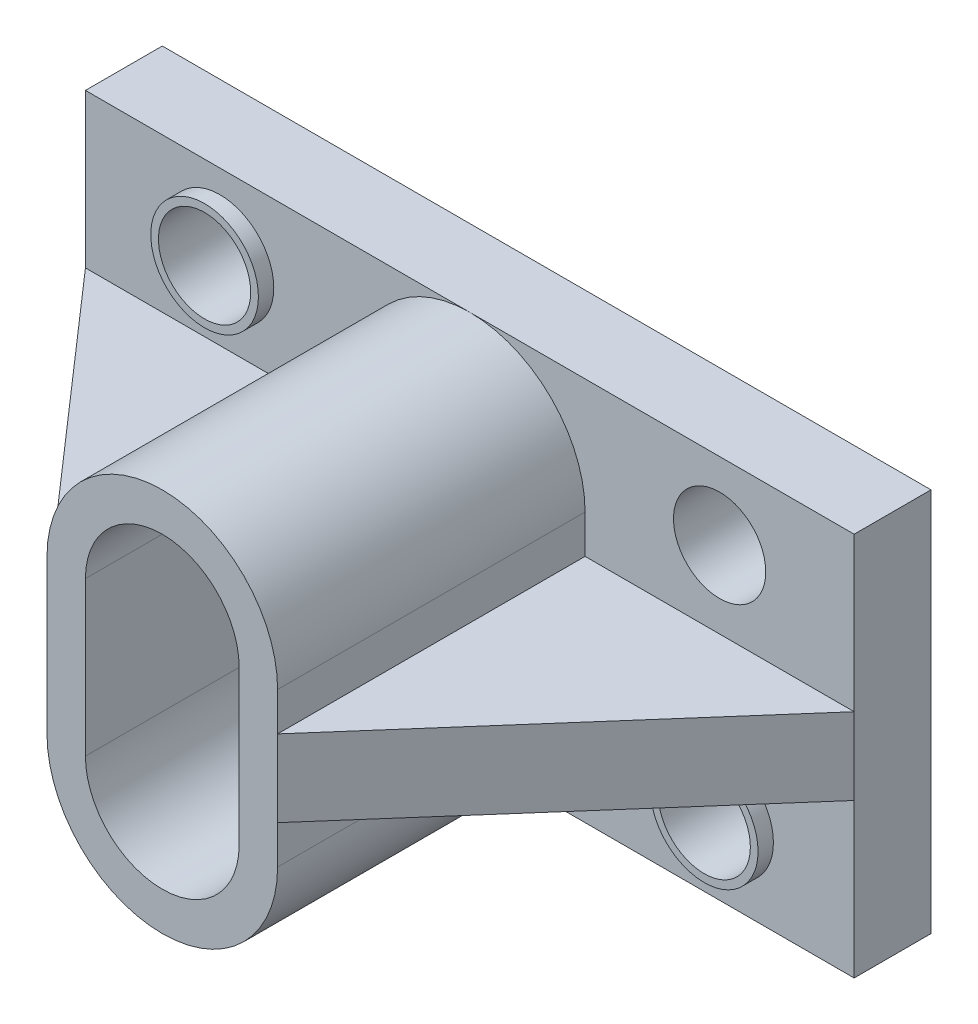
ISO-10303-21;
HEADER;
FILE_DESCRIPTION(('STEP AP214'),'2;1');
FILE_NAME('part.step','',(''),(''),'','','');
FILE_SCHEMA(('AUTOMOTIVE_DESIGN { 1 0 10303 214 1 1 1 1 }'));
ENDSEC;
DATA;
#1=APPLICATION_CONTEXT('core data for automotive mechanical design processes');
#2=APPLICATION_PROTOCOL_DEFINITION('international standard','automotive_design',2000,#1);
#3=PRODUCT_CONTEXT('',#1,'mechanical');
#4=PRODUCT('Part','Part','',(#3));
#5=PRODUCT_RELATED_PRODUCT_CATEGORY('part','',(#4));
#6=PRODUCT_DEFINITION_FORMATION('','',#4);
#7=PRODUCT_DEFINITION_CONTEXT('part definition',#1,'design');
#8=PRODUCT_DEFINITION('design','',#6,#7);
#9=PRODUCT_DEFINITION_SHAPE('','',#8);
#10=(LENGTH_UNIT() NAMED_UNIT(*) SI_UNIT(.MILLI.,.METRE.));
#11=(NAMED_UNIT(*) PLANE_ANGLE_UNIT() SI_UNIT($,.RADIAN.));
#12=(NAMED_UNIT(*) SI_UNIT($,.STERADIAN.) SOLID_ANGLE_UNIT());
#13=UNCERTAINTY_MEASURE_WITH_UNIT(LENGTH_MEASURE(1.E-05),#10,'distance_accuracy_value','');
#14=(GEOMETRIC_REPRESENTATION_CONTEXT(3) GLOBAL_UNCERTAINTY_ASSIGNED_CONTEXT((#13)) GLOBAL_UNIT_ASSIGNED_CONTEXT((#10,
#11,#12)) REPRESENTATION_CONTEXT('',''));
#15=CARTESIAN_POINT('',(0.,0.,0.));
#16=DIRECTION('',(0.,0.,1.));
#17=DIRECTION('',(1.,0.,0.));
#18=AXIS2_PLACEMENT_3D('',#15,#16,#17);
#19=CARTESIAN_POINT('',(0.,0.,10.));
#20=DIRECTION('',(0.,0.,1.));
#21=DIRECTION('',(1.,0.,0.));
#22=AXIS2_PLACEMENT_3D('',#19,#20,#21);
#23=PLANE('',#22);
#24=CARTESIAN_POINT('',(17.5,10.,10.));
#25=DIRECTION('',(0.,0.,1.));
#26=DIRECTION('',(1.,0.,0.));
#27=AXIS2_PLACEMENT_3D('',#24,#25,#26);
#28=CIRCLE('',#27,7.);
#29=CARTESIAN_POINT('',(24.5,10.,10.));
#30=VERTEX_POINT('',#29);
#31=EDGE_CURVE('E278',#30,#30,#28,.T.);
#32=ORIENTED_EDGE('',*,*,#31,.F.);
#33=EDGE_LOOP('',(#32));
#34=FACE_BOUND('',#33,.T.);
#35=DIRECTION('',(0.,-1.,0.));
#36=VECTOR('',#35,1.);
#37=CARTESIAN_POINT('',(35.,15.,10.));
#38=LINE('',#37,#36);
#39=CARTESIAN_POINT('',(35.,20.,10.));
#40=VERTEX_POINT('',#39);
#41=CARTESIAN_POINT('',(35.,15.,10.));
#42=VERTEX_POINT('',#41);
#43=EDGE_CURVE('E380',#40,#42,#38,.T.);
#44=ORIENTED_EDGE('',*,*,#43,.F.);
#45=DIRECTION('',(-1.,0.,0.));
#46=VECTOR('',#45,1.);
#47=CARTESIAN_POINT('',(0.,20.,10.));
#48=LINE('',#47,#46);
#49=CARTESIAN_POINT('',(0.,20.,10.));
#50=VERTEX_POINT('',#49);
#51=EDGE_CURVE('E72',#40,#50,#48,.T.);
#52=ORIENTED_EDGE('',*,*,#51,.T.);
#53=DIRECTION('',(0.,-1.,0.));
#54=VECTOR('',#53,1.);
#55=CARTESIAN_POINT('',(0.,50.,10.));
#56=LINE('',#55,#54);
#57=CARTESIAN_POINT('',(0.,0.,10.));
#58=VERTEX_POINT('',#57);
#59=EDGE_CURVE('E397',#50,#58,#56,.T.);
#60=ORIENTED_EDGE('',*,*,#59,.T.);
#61=DIRECTION('',(1.,0.,0.));
#62=VECTOR('',#61,1.);
#63=CARTESIAN_POINT('',(0.,0.,10.));
#64=LINE('',#63,#62);
#65=CARTESIAN_POINT('',(50.,0.,10.));
#66=VERTEX_POINT('',#65);
#67=EDGE_CURVE('E399',#58,#66,#64,.T.);
#68=ORIENTED_EDGE('',*,*,#67,.T.);
#69=CARTESIAN_POINT('',(50.,15.,10.));
#70=DIRECTION('',(0.,0.,1.));
#71=DIRECTION('',(1.,0.,0.));
#72=AXIS2_PLACEMENT_3D('',#69,#70,#71);
#73=CIRCLE('',#72,15.);
#74=EDGE_CURVE('E355',#42,#66,#73,.T.);
#75=ORIENTED_EDGE('',*,*,#74,.F.);
#76=EDGE_LOOP('',(#44,#52,#60,#68,#75));
#77=FACE_BOUND('',#76,.T.);
#78=ADVANCED_FACE('F44',(#34,#77),#23,.T.);
#79=CARTESIAN_POINT('',(35.,15.,50.));
#80=DIRECTION('',(1.,0.,0.));
#81=DIRECTION('',(0.,0.,-1.));
#82=AXIS2_PLACEMENT_3D('',#79,#80,#81);
#83=PLANE('',#82);
#84=DIRECTION('',(0.,0.,1.));
#85=VECTOR('',#84,1.);
#86=CARTESIAN_POINT('',(35.,20.,50.));
#87=LINE('',#86,#85);
#88=CARTESIAN_POINT('',(35.,20.,50.));
#89=VERTEX_POINT('',#88);
#90=EDGE_CURVE('E288',#40,#89,#87,.T.);
#91=ORIENTED_EDGE('',*,*,#90,.F.);
#92=ORIENTED_EDGE('',*,*,#43,.T.);
#93=DIRECTION('',(0.,0.,-1.));
#94=VECTOR('',#93,1.);
#95=CARTESIAN_POINT('',(35.,15.,50.));
#96=LINE('',#95,#94);
#97=CARTESIAN_POINT('',(35.,15.,50.));
#98=VERTEX_POINT('',#97);
#99=EDGE_CURVE('E367',#98,#42,#96,.T.);
#100=ORIENTED_EDGE('',*,*,#99,.F.);
#101=DIRECTION('',(0.,-1.,0.));
#102=VECTOR('',#101,1.);
#103=CARTESIAN_POINT('',(35.,15.,50.));
#104=LINE('',#103,#102);
#105=EDGE_CURVE('E362',#89,#98,#104,.T.);
#106=ORIENTED_EDGE('',*,*,#105,.F.);
#107=EDGE_LOOP('',(#91,#92,#100,#106));
#108=FACE_BOUND('',#107,.T.);
#109=ADVANCED_FACE('F450',(#108),#83,.F.);
#110=CARTESIAN_POINT('',(82.5,10.,10.));
#111=DIRECTION('',(0.,0.,1.));
#112=DIRECTION('',(1.,0.,0.));
#113=AXIS2_PLACEMENT_3D('',#110,#111,#112);
#114=CIRCLE('',#113,7.);
#115=CARTESIAN_POINT('',(89.5,10.,10.));
#116=VERTEX_POINT('',#115);
#117=EDGE_CURVE('E272',#116,#116,#114,.T.);
#118=ORIENTED_EDGE('',*,*,#117,.F.);
#119=EDGE_LOOP('',(#118));
#120=FACE_BOUND('',#119,.T.);
#121=DIRECTION('',(0.,1.,0.));
#122=VECTOR('',#121,1.);
#123=CARTESIAN_POINT('',(100.,0.,10.));
#124=LINE('',#123,#122);
#125=CARTESIAN_POINT('',(100.,0.,10.));
#126=VERTEX_POINT('',#125);
#127=CARTESIAN_POINT('',(100.,20.,10.));
#128=VERTEX_POINT('',#127);
#129=EDGE_CURVE('E402',#126,#128,#124,.T.);
#130=ORIENTED_EDGE('',*,*,#129,.T.);
#131=DIRECTION('',(-1.,0.,0.));
#132=VECTOR('',#131,1.);
#133=CARTESIAN_POINT('',(0.,20.,10.));
#134=LINE('',#133,#132);
#135=CARTESIAN_POINT('',(65.,20.,10.));
#136=VERTEX_POINT('',#135);
#137=EDGE_CURVE('E312',#128,#136,#134,.T.);
#138=ORIENTED_EDGE('',*,*,#137,.T.);
#139=DIRECTION('',(0.,1.,0.));
#140=VECTOR('',#139,1.);
#141=CARTESIAN_POINT('',(65.,15.,10.));
#142=LINE('',#141,#140);
#143=CARTESIAN_POINT('',(65.,15.,10.));
#144=VERTEX_POINT('',#143);
#145=EDGE_CURVE('E372',#144,#136,#142,.T.);
#146=ORIENTED_EDGE('',*,*,#145,.F.);
#147=EDGE_CURVE('E53',#66,#144,#73,.T.);
#148=ORIENTED_EDGE('',*,*,#147,.F.);
#149=EDGE_CURVE('E394',#66,#126,#64,.T.);
#150=ORIENTED_EDGE('',*,*,#149,.T.);
#151=EDGE_LOOP('',(#130,#138,#146,#148,#150));
#152=FACE_BOUND('',#151,.T.);
#153=ADVANCED_FACE('F458',(#120,#152),#23,.T.);
#154=CARTESIAN_POINT('',(65.,15.,50.));
#155=DIRECTION('',(-1.,0.,0.));
#156=DIRECTION('',(0.,0.,1.));
#157=AXIS2_PLACEMENT_3D('',#154,#155,#156);
#158=PLANE('',#157);
#159=DIRECTION('',(0.,0.,-1.));
#160=VECTOR('',#159,1.);
#161=CARTESIAN_POINT('',(65.,20.,50.));
#162=LINE('',#161,#160);
#163=CARTESIAN_POINT('',(65.,20.,50.));
#164=VERTEX_POINT('',#163);
#165=EDGE_CURVE('E308',#164,#136,#162,.T.);
#166=ORIENTED_EDGE('',*,*,#165,.F.);
#167=DIRECTION('',(0.,1.,0.));
#168=VECTOR('',#167,1.);
#169=CARTESIAN_POINT('',(65.,15.,50.));
#170=LINE('',#169,#168);
#171=CARTESIAN_POINT('',(65.,15.,50.));
#172=VERTEX_POINT('',#171);
#173=EDGE_CURVE('E360',#172,#164,#170,.T.);
#174=ORIENTED_EDGE('',*,*,#173,.F.);
#175=DIRECTION('',(0.,0.,-1.));
#176=VECTOR('',#175,1.);
#177=CARTESIAN_POINT('',(65.,15.,50.));
#178=LINE('',#177,#176);
#179=EDGE_CURVE('E389',#172,#144,#178,.T.);
#180=ORIENTED_EDGE('',*,*,#179,.T.);
#181=ORIENTED_EDGE('',*,*,#145,.T.);
#182=EDGE_LOOP('',(#166,#174,#180,#181));
#183=FACE_BOUND('',#182,.T.);
#184=ADVANCED_FACE('F437',(#183),#158,.F.);
#185=CARTESIAN_POINT('',(17.5,40.,10.));
#186=DIRECTION('',(0.,0.,1.));
#187=DIRECTION('',(1.,0.,0.));
#188=AXIS2_PLACEMENT_3D('',#185,#186,#187);
#189=CIRCLE('',#188,7.);
#190=CARTESIAN_POINT('',(24.5,40.,10.));
#191=VERTEX_POINT('',#190);
#192=EDGE_CURVE('E265',#191,#191,#189,.T.);
#193=ORIENTED_EDGE('',*,*,#192,.F.);
#194=EDGE_LOOP('',(#193));
#195=FACE_BOUND('',#194,.T.);
#196=DIRECTION('',(-1.,0.,0.));
#197=VECTOR('',#196,1.);
#198=CARTESIAN_POINT('',(0.,30.,10.));
#199=LINE('',#198,#197);
#200=CARTESIAN_POINT('',(35.,30.,10.));
#201=VERTEX_POINT('',#200);
#202=CARTESIAN_POINT('',(0.,30.,10.));
#203=VERTEX_POINT('',#202);
#204=EDGE_CURVE('E298',#201,#203,#199,.T.);
#205=ORIENTED_EDGE('',*,*,#204,.F.);
#206=CARTESIAN_POINT('',(35.,35.,10.));
#207=VERTEX_POINT('',#206);
#208=EDGE_CURVE('E356',#207,#201,#38,.T.);
#209=ORIENTED_EDGE('',*,*,#208,.F.);
#210=CARTESIAN_POINT('',(50.,35.,10.));
#211=DIRECTION('',(0.,0.,1.));
#212=DIRECTION('',(1.,0.,0.));
#213=AXIS2_PLACEMENT_3D('',#210,#211,#212);
#214=CIRCLE('',#213,15.);
#215=CARTESIAN_POINT('',(50.,50.,10.));
#216=VERTEX_POINT('',#215);
#217=EDGE_CURVE('E11',#216,#207,#214,.T.);
#218=ORIENTED_EDGE('',*,*,#217,.F.);
#219=DIRECTION('',(-1.,0.,0.));
#220=VECTOR('',#219,1.);
#221=CARTESIAN_POINT('',(100.,50.,10.));
#222=LINE('',#221,#220);
#223=CARTESIAN_POINT('',(0.,50.,10.));
#224=VERTEX_POINT('',#223);
#225=EDGE_CURVE('E404',#216,#224,#222,.T.);
#226=ORIENTED_EDGE('',*,*,#225,.T.);
#227=EDGE_CURVE('E395',#224,#203,#56,.T.);
#228=ORIENTED_EDGE('',*,*,#227,.T.);
#229=EDGE_LOOP('',(#205,#209,#218,#226,#228));
#230=FACE_BOUND('',#229,.T.);
#231=ADVANCED_FACE('F486',(#195,#230),#23,.T.);
#232=CARTESIAN_POINT('',(0.,50.,10.));
#233=DIRECTION('',(1.,0.,0.));
#234=DIRECTION('',(0.,0.,-1.));
#235=AXIS2_PLACEMENT_3D('',#232,#233,#234);
#236=PLANE('',#235);
#237=DIRECTION('',(0.,-1.,0.));
#238=VECTOR('',#237,1.);
#239=CARTESIAN_POINT('',(0.,50.,0.));
#240=LINE('',#239,#238);
#241=CARTESIAN_POINT('',(0.,50.,0.));
#242=VERTEX_POINT('',#241);
#243=CARTESIAN_POINT('',(0.,0.,0.));
#244=VERTEX_POINT('',#243);
#245=EDGE_CURVE('E391',#242,#244,#240,.T.);
#246=ORIENTED_EDGE('',*,*,#245,.T.);
#247=DIRECTION('',(0.,0.,-1.));
#248=VECTOR('',#247,1.);
#249=CARTESIAN_POINT('',(0.,0.,10.));
#250=LINE('',#249,#248);
#251=EDGE_CURVE('E47',#58,#244,#250,.T.);
#252=ORIENTED_EDGE('',*,*,#251,.F.);
#253=ORIENTED_EDGE('',*,*,#59,.F.);
#254=DIRECTION('',(0.,1.,0.));
#255=VECTOR('',#254,1.);
#256=CARTESIAN_POINT('',(0.,50.,9.99999999999999));
#257=LINE('',#256,#255);
#258=EDGE_CURVE('E301',#203,#50,#257,.F.);
#259=ORIENTED_EDGE('',*,*,#258,.F.);
#260=ORIENTED_EDGE('',*,*,#227,.F.);
#261=DIRECTION('',(0.,0.,-1.));
#262=VECTOR('',#261,1.);
#263=CARTESIAN_POINT('',(0.,50.,10.));
#264=LINE('',#263,#262);
#265=EDGE_CURVE('E409',#224,#242,#264,.T.);
#266=ORIENTED_EDGE('',*,*,#265,.T.);
#267=EDGE_LOOP('',(#246,#252,#253,#259,#260,#266));
#268=FACE_BOUND('',#267,.T.);
#269=ADVANCED_FACE('F50',(#268),#236,.F.);
#270=CARTESIAN_POINT('',(0.,0.,10.));
#271=DIRECTION('',(0.,1.,0.));
#272=DIRECTION('',(0.,0.,1.));
#273=AXIS2_PLACEMENT_3D('',#270,#271,#272);
#274=PLANE('',#273);
#275=DIRECTION('',(1.,0.,0.));
#276=VECTOR('',#275,1.);
#277=CARTESIAN_POINT('',(0.,0.,0.));
#278=LINE('',#277,#276);
#279=CARTESIAN_POINT('',(100.,0.,0.));
#280=VERTEX_POINT('',#279);
#281=EDGE_CURVE('E408',#244,#280,#278,.T.);
#282=ORIENTED_EDGE('',*,*,#281,.T.);
#283=DIRECTION('',(0.,0.,-1.));
#284=VECTOR('',#283,1.);
#285=CARTESIAN_POINT('',(100.,0.,10.));
#286=LINE('',#285,#284);
#287=EDGE_CURVE('E418',#126,#280,#286,.T.);
#288=ORIENTED_EDGE('',*,*,#287,.F.);
#289=ORIENTED_EDGE('',*,*,#149,.F.);
#290=ORIENTED_EDGE('',*,*,#67,.F.);
#291=ORIENTED_EDGE('',*,*,#251,.T.);
#292=EDGE_LOOP('',(#282,#288,#289,#290,#291));
#293=FACE_BOUND('',#292,.T.);
#294=ADVANCED_FACE('F449',(#293),#274,.F.);
#295=CARTESIAN_POINT('',(100.,0.,10.));
#296=DIRECTION('',(-1.,0.,0.));
#297=DIRECTION('',(0.,0.,1.));
#298=AXIS2_PLACEMENT_3D('',#295,#296,#297);
#299=PLANE('',#298);
#300=CARTESIAN_POINT('',(100.,30.,10.));
#301=VERTEX_POINT('',#300);
#302=CARTESIAN_POINT('',(100.,50.,10.));
#303=VERTEX_POINT('',#302);
#304=EDGE_CURVE('E398',#301,#303,#124,.T.);
#305=ORIENTED_EDGE('',*,*,#304,.F.);
#306=DIRECTION('',(0.,1.,0.));
#307=VECTOR('',#306,1.);
#308=CARTESIAN_POINT('',(100.,0.,10.));
#309=LINE('',#308,#307);
#310=EDGE_CURVE('E322',#128,#301,#309,.T.);
#311=ORIENTED_EDGE('',*,*,#310,.F.);
#312=ORIENTED_EDGE('',*,*,#129,.F.);
#313=ORIENTED_EDGE('',*,*,#287,.T.);
#314=DIRECTION('',(0.,1.,0.));
#315=VECTOR('',#314,1.);
#316=CARTESIAN_POINT('',(100.,0.,0.));
#317=LINE('',#316,#315);
#318=CARTESIAN_POINT('',(100.,50.,0.));
#319=VERTEX_POINT('',#318);
#320=EDGE_CURVE('E415',#280,#319,#317,.T.);
#321=ORIENTED_EDGE('',*,*,#320,.T.);
#322=DIRECTION('',(0.,0.,-1.));
#323=VECTOR('',#322,1.);
#324=CARTESIAN_POINT('',(100.,50.,10.));
#325=LINE('',#324,#323);
#326=EDGE_CURVE('E420',#303,#319,#325,.T.);
#327=ORIENTED_EDGE('',*,*,#326,.F.);
#328=EDGE_LOOP('',(#305,#311,#312,#313,#321,#327));
#329=FACE_BOUND('',#328,.T.);
#330=ADVANCED_FACE('F460',(#329),#299,.F.);
#331=CARTESIAN_POINT('',(100.,50.,10.));
#332=DIRECTION('',(0.,-1.,0.));
#333=DIRECTION('',(0.,0.,-1.));
#334=AXIS2_PLACEMENT_3D('',#331,#332,#333);
#335=PLANE('',#334);
#336=DIRECTION('',(-1.,0.,0.));
#337=VECTOR('',#336,1.);
#338=CARTESIAN_POINT('',(100.,50.,0.));
#339=LINE('',#338,#337);
#340=EDGE_CURVE('E413',#319,#242,#339,.T.);
#341=ORIENTED_EDGE('',*,*,#340,.T.);
#342=ORIENTED_EDGE('',*,*,#265,.F.);
#343=ORIENTED_EDGE('',*,*,#225,.F.);
#344=EDGE_CURVE('E403',#303,#216,#222,.T.);
#345=ORIENTED_EDGE('',*,*,#344,.F.);
#346=ORIENTED_EDGE('',*,*,#326,.T.);
#347=EDGE_LOOP('',(#341,#342,#343,#345,#346));
#348=FACE_BOUND('',#347,.T.);
#349=ADVANCED_FACE('F516',(#348),#335,.F.);
#350=CARTESIAN_POINT('',(82.5,40.,10.));
#351=DIRECTION('',(0.,0.,1.));
#352=DIRECTION('',(1.,0.,0.));
#353=AXIS2_PLACEMENT_3D('',#350,#351,#352);
#354=CIRCLE('',#353,6.);
#355=CARTESIAN_POINT('',(88.5,40.,10.));
#356=VERTEX_POINT('',#355);
#357=EDGE_CURVE('E249',#356,#356,#354,.T.);
#358=ORIENTED_EDGE('',*,*,#357,.F.);
#359=EDGE_LOOP('',(#358));
#360=FACE_BOUND('',#359,.T.);
#361=DIRECTION('',(-1.,0.,0.));
#362=VECTOR('',#361,1.);
#363=CARTESIAN_POINT('',(0.,30.,10.));
#364=LINE('',#363,#362);
#365=CARTESIAN_POINT('',(65.,30.,10.));
#366=VERTEX_POINT('',#365);
#367=EDGE_CURVE('E319',#301,#366,#364,.T.);
#368=ORIENTED_EDGE('',*,*,#367,.F.);
#369=ORIENTED_EDGE('',*,*,#304,.T.);
#370=ORIENTED_EDGE('',*,*,#344,.T.);
#371=CARTESIAN_POINT('',(65.,35.,10.));
#372=VERTEX_POINT('',#371);
#373=EDGE_CURVE('E57',#372,#216,#214,.T.);
#374=ORIENTED_EDGE('',*,*,#373,.F.);
#375=EDGE_CURVE('E373',#366,#372,#142,.T.);
#376=ORIENTED_EDGE('',*,*,#375,.F.);
#377=EDGE_LOOP('',(#368,#369,#370,#374,#376));
#378=FACE_BOUND('',#377,.T.);
#379=ADVANCED_FACE('F507',(#360,#378),#23,.T.);
#380=CARTESIAN_POINT('',(0.,0.,0.));
#381=DIRECTION('',(0.,0.,1.));
#382=DIRECTION('',(1.,0.,0.));
#383=AXIS2_PLACEMENT_3D('',#380,#381,#382);
#384=PLANE('',#383);
#385=DIRECTION('',(0.,-1.,0.));
#386=VECTOR('',#385,1.);
#387=CARTESIAN_POINT('',(39.9346471149662,15.,0.));
#388=LINE('',#387,#386);
#389=CARTESIAN_POINT('',(39.9346471149662,35.,0.));
#390=VERTEX_POINT('',#389);
#391=CARTESIAN_POINT('',(39.9346471149662,15.,0.));
#392=VERTEX_POINT('',#391);
#393=EDGE_CURVE('E216',#390,#392,#388,.T.);
#394=ORIENTED_EDGE('',*,*,#393,.T.);
#395=CARTESIAN_POINT('',(50.,15.,0.));
#396=DIRECTION('',(0.,0.,1.));
#397=DIRECTION('',(1.,0.,0.));
#398=AXIS2_PLACEMENT_3D('',#395,#396,#397);
#399=CIRCLE('',#398,10.0653528850339);
#400=CARTESIAN_POINT('',(60.0653528850339,15.,0.));
#401=VERTEX_POINT('',#400);
#402=EDGE_CURVE('E206',#392,#401,#399,.T.);
#403=ORIENTED_EDGE('',*,*,#402,.T.);
#404=DIRECTION('',(0.,1.,0.));
#405=VECTOR('',#404,1.);
#406=CARTESIAN_POINT('',(60.0653528850339,15.,0.));
#407=LINE('',#406,#405);
#408=CARTESIAN_POINT('',(60.0653528850339,35.,0.));
#409=VERTEX_POINT('',#408);
#410=EDGE_CURVE('E218',#401,#409,#407,.T.);
#411=ORIENTED_EDGE('',*,*,#410,.T.);
#412=CARTESIAN_POINT('',(50.,35.,0.));
#413=DIRECTION('',(0.,0.,1.));
#414=DIRECTION('',(1.,0.,0.));
#415=AXIS2_PLACEMENT_3D('',#412,#413,#414);
#416=CIRCLE('',#415,10.0653528850339);
#417=EDGE_CURVE('E64',#409,#390,#416,.T.);
#418=ORIENTED_EDGE('',*,*,#417,.T.);
#419=EDGE_LOOP('',(#394,#403,#411,#418));
#420=FACE_BOUND('',#419,.T.);
#421=CARTESIAN_POINT('',(82.5,10.,0.));
#422=DIRECTION('',(0.,0.,1.));
#423=DIRECTION('',(1.,0.,0.));
#424=AXIS2_PLACEMENT_3D('',#421,#422,#423);
#425=CIRCLE('',#424,6.);
#426=CARTESIAN_POINT('',(88.5,10.,0.));
#427=VERTEX_POINT('',#426);
#428=EDGE_CURVE('E241',#427,#427,#425,.T.);
#429=ORIENTED_EDGE('',*,*,#428,.T.);
#430=EDGE_LOOP('',(#429));
#431=FACE_BOUND('',#430,.T.);
#432=CARTESIAN_POINT('',(82.5,40.,0.));
#433=DIRECTION('',(0.,0.,1.));
#434=DIRECTION('',(1.,0.,0.));
#435=AXIS2_PLACEMENT_3D('',#432,#433,#434);
#436=CIRCLE('',#435,6.);
#437=CARTESIAN_POINT('',(88.5,40.,0.));
#438=VERTEX_POINT('',#437);
#439=EDGE_CURVE('E250',#438,#438,#436,.T.);
#440=ORIENTED_EDGE('',*,*,#439,.T.);
#441=EDGE_LOOP('',(#440));
#442=FACE_BOUND('',#441,.T.);
#443=CARTESIAN_POINT('',(17.5,10.,0.));
#444=DIRECTION('',(0.,0.,1.));
#445=DIRECTION('',(1.,0.,0.));
#446=AXIS2_PLACEMENT_3D('',#443,#444,#445);
#447=CIRCLE('',#446,6.);
#448=CARTESIAN_POINT('',(23.5,10.,0.));
#449=VERTEX_POINT('',#448);
#450=EDGE_CURVE('E254',#449,#449,#447,.T.);
#451=ORIENTED_EDGE('',*,*,#450,.T.);
#452=EDGE_LOOP('',(#451));
#453=FACE_BOUND('',#452,.T.);
#454=CARTESIAN_POINT('',(17.5,40.,0.));
#455=DIRECTION('',(0.,0.,1.));
#456=DIRECTION('',(1.,0.,0.));
#457=AXIS2_PLACEMENT_3D('',#454,#455,#456);
#458=CIRCLE('',#457,6.);
#459=CARTESIAN_POINT('',(23.5,40.,0.));
#460=VERTEX_POINT('',#459);
#461=EDGE_CURVE('E257',#460,#460,#458,.T.);
#462=ORIENTED_EDGE('',*,*,#461,.T.);
#463=EDGE_LOOP('',(#462));
#464=FACE_BOUND('',#463,.T.);
#465=ORIENTED_EDGE('',*,*,#340,.F.);
#466=ORIENTED_EDGE('',*,*,#320,.F.);
#467=ORIENTED_EDGE('',*,*,#281,.F.);
#468=ORIENTED_EDGE('',*,*,#245,.F.);
#469=EDGE_LOOP('',(#465,#466,#467,#468));
#470=FACE_BOUND('',#469,.T.);
#471=ADVANCED_FACE('F225',(#420,#431,#442,#453,#464,#470),#384,.F.);
#472=CARTESIAN_POINT('',(50.,15.,50.));
#473=DIRECTION('',(0.,0.,1.));
#474=DIRECTION('',(1.,0.,0.));
#475=AXIS2_PLACEMENT_3D('',#472,#473,#474);
#476=PLANE('',#475);
#477=CARTESIAN_POINT('',(50.,35.,50.));
#478=DIRECTION('',(0.,0.,1.));
#479=DIRECTION('',(1.,0.,0.));
#480=AXIS2_PLACEMENT_3D('',#477,#478,#479);
#481=CIRCLE('',#480,10.);
#482=CARTESIAN_POINT('',(60.,35.,50.));
#483=VERTEX_POINT('',#482);
#484=CARTESIAN_POINT('',(40.,35.,50.));
#485=VERTEX_POINT('',#484);
#486=EDGE_CURVE('E329',#483,#485,#481,.T.);
#487=ORIENTED_EDGE('',*,*,#486,.F.);
#488=DIRECTION('',(0.,1.,0.));
#489=VECTOR('',#488,1.);
#490=CARTESIAN_POINT('',(60.,15.,50.));
#491=LINE('',#490,#489);
#492=CARTESIAN_POINT('',(60.,15.,50.));
#493=VERTEX_POINT('',#492);
#494=EDGE_CURVE('E330',#493,#483,#491,.T.);
#495=ORIENTED_EDGE('',*,*,#494,.F.);
#496=CARTESIAN_POINT('',(50.,15.,50.));
#497=DIRECTION('',(0.,0.,1.));
#498=DIRECTION('',(1.,0.,0.));
#499=AXIS2_PLACEMENT_3D('',#496,#497,#498);
#500=CIRCLE('',#499,10.);
#501=CARTESIAN_POINT('',(40.,15.,50.));
#502=VERTEX_POINT('',#501);
#503=EDGE_CURVE('E323',#502,#493,#500,.T.);
#504=ORIENTED_EDGE('',*,*,#503,.F.);
#505=DIRECTION('',(0.,-1.,0.));
#506=VECTOR('',#505,1.);
#507=CARTESIAN_POINT('',(40.,15.,50.));
#508=LINE('',#507,#506);
#509=EDGE_CURVE('E335',#485,#502,#508,.T.);
#510=ORIENTED_EDGE('',*,*,#509,.F.);
#511=EDGE_LOOP('',(#487,#495,#504,#510));
#512=FACE_BOUND('',#511,.T.);
#513=CARTESIAN_POINT('',(65.,30.,50.));
#514=VERTEX_POINT('',#513);
#515=EDGE_CURVE('E361',#164,#514,#170,.T.);
#516=ORIENTED_EDGE('',*,*,#515,.T.);
#517=CARTESIAN_POINT('',(65.,35.,50.));
#518=VERTEX_POINT('',#517);
#519=EDGE_CURVE('E357',#514,#518,#170,.T.);
#520=ORIENTED_EDGE('',*,*,#519,.T.);
#521=CARTESIAN_POINT('',(50.,35.,50.));
#522=DIRECTION('',(0.,0.,1.));
#523=DIRECTION('',(1.,0.,0.));
#524=AXIS2_PLACEMENT_3D('',#521,#522,#523);
#525=CIRCLE('',#524,15.);
#526=CARTESIAN_POINT('',(35.,35.,50.));
#527=VERTEX_POINT('',#526);
#528=EDGE_CURVE('E365',#518,#527,#525,.T.);
#529=ORIENTED_EDGE('',*,*,#528,.T.);
#530=CARTESIAN_POINT('',(35.,30.,50.));
#531=VERTEX_POINT('',#530);
#532=EDGE_CURVE('E366',#527,#531,#104,.T.);
#533=ORIENTED_EDGE('',*,*,#532,.T.);
#534=EDGE_CURVE('E369',#531,#89,#104,.T.);
#535=ORIENTED_EDGE('',*,*,#534,.T.);
#536=ORIENTED_EDGE('',*,*,#105,.T.);
#537=CARTESIAN_POINT('',(50.,15.,50.));
#538=DIRECTION('',(0.,0.,1.));
#539=DIRECTION('',(1.,0.,0.));
#540=AXIS2_PLACEMENT_3D('',#537,#538,#539);
#541=CIRCLE('',#540,15.);
#542=EDGE_CURVE('E351',#98,#172,#541,.T.);
#543=ORIENTED_EDGE('',*,*,#542,.T.);
#544=ORIENTED_EDGE('',*,*,#173,.T.);
#545=EDGE_LOOP('',(#516,#520,#529,#533,#535,#536,#543,#544));
#546=FACE_BOUND('',#545,.T.);
#547=ADVANCED_FACE('F442',(#512,#546),#476,.T.);
#548=CARTESIAN_POINT('',(50.,15.,50.));
#549=DIRECTION('',(0.,0.,-1.));
#550=DIRECTION('',(-1.,0.,0.));
#551=AXIS2_PLACEMENT_3D('',#548,#549,#550);
#552=CYLINDRICAL_SURFACE('',#551,15.);
#553=ORIENTED_EDGE('',*,*,#74,.T.);
#554=ORIENTED_EDGE('',*,*,#147,.T.);
#555=ORIENTED_EDGE('',*,*,#179,.F.);
#556=ORIENTED_EDGE('',*,*,#542,.F.);
#557=ORIENTED_EDGE('',*,*,#99,.T.);
#558=EDGE_LOOP('',(#553,#554,#555,#556,#557));
#559=FACE_BOUND('',#558,.T.);
#560=ADVANCED_FACE('F433',(#559),#552,.T.);
#561=ORIENTED_EDGE('',*,*,#519,.F.);
#562=DIRECTION('',(0.,0.,-1.));
#563=VECTOR('',#562,1.);
#564=CARTESIAN_POINT('',(65.,30.,50.));
#565=LINE('',#564,#563);
#566=EDGE_CURVE('E317',#514,#366,#565,.T.);
#567=ORIENTED_EDGE('',*,*,#566,.T.);
#568=ORIENTED_EDGE('',*,*,#375,.T.);
#569=DIRECTION('',(0.,0.,-1.));
#570=VECTOR('',#569,1.);
#571=CARTESIAN_POINT('',(65.,35.,50.));
#572=LINE('',#571,#570);
#573=EDGE_CURVE('E383',#518,#372,#572,.T.);
#574=ORIENTED_EDGE('',*,*,#573,.F.);
#575=EDGE_LOOP('',(#561,#567,#568,#574));
#576=FACE_BOUND('',#575,.T.);
#577=ADVANCED_FACE('F472',(#576),#158,.F.);
#578=CARTESIAN_POINT('',(50.,35.,50.));
#579=DIRECTION('',(0.,0.,-1.));
#580=DIRECTION('',(-1.,0.,0.));
#581=AXIS2_PLACEMENT_3D('',#578,#579,#580);
#582=CYLINDRICAL_SURFACE('',#581,15.);
#583=ORIENTED_EDGE('',*,*,#373,.T.);
#584=ORIENTED_EDGE('',*,*,#217,.T.);
#585=DIRECTION('',(0.,0.,-1.));
#586=VECTOR('',#585,1.);
#587=CARTESIAN_POINT('',(35.,35.,50.));
#588=LINE('',#587,#586);
#589=EDGE_CURVE('E385',#527,#207,#588,.T.);
#590=ORIENTED_EDGE('',*,*,#589,.F.);
#591=ORIENTED_EDGE('',*,*,#528,.F.);
#592=ORIENTED_EDGE('',*,*,#573,.T.);
#593=EDGE_LOOP('',(#583,#584,#590,#591,#592));
#594=FACE_BOUND('',#593,.T.);
#595=ADVANCED_FACE('F473',(#594),#582,.T.);
#596=ORIENTED_EDGE('',*,*,#208,.T.);
#597=DIRECTION('',(0.,0.,1.));
#598=VECTOR('',#597,1.);
#599=CARTESIAN_POINT('',(35.,30.,50.));
#600=LINE('',#599,#598);
#601=EDGE_CURVE('E299',#201,#531,#600,.T.);
#602=ORIENTED_EDGE('',*,*,#601,.T.);
#603=ORIENTED_EDGE('',*,*,#532,.F.);
#604=ORIENTED_EDGE('',*,*,#589,.T.);
#605=EDGE_LOOP('',(#596,#602,#603,#604));
#606=FACE_BOUND('',#605,.T.);
#607=ADVANCED_FACE('F477',(#606),#83,.F.);
#608=CARTESIAN_POINT('',(50.,15.,50.));
#609=DIRECTION('',(0.,0.,-1.));
#610=DIRECTION('',(-1.,0.,0.));
#611=AXIS2_PLACEMENT_3D('',#608,#609,#610);
#612=CYLINDRICAL_SURFACE('',#611,10.);
#613=CARTESIAN_POINT('',(50.,15.,10.));
#614=DIRECTION('',(0.,0.,1.));
#615=DIRECTION('',(1.,0.,0.));
#616=AXIS2_PLACEMENT_3D('',#613,#614,#615);
#617=CIRCLE('',#616,10.);
#618=CARTESIAN_POINT('',(40.,15.,10.));
#619=VERTEX_POINT('',#618);
#620=CARTESIAN_POINT('',(60.,15.,10.));
#621=VERTEX_POINT('',#620);
#622=EDGE_CURVE('E321',#619,#621,#617,.T.);
#623=ORIENTED_EDGE('',*,*,#622,.F.);
#624=DIRECTION('',(0.,0.,-1.));
#625=VECTOR('',#624,1.);
#626=CARTESIAN_POINT('',(40.,15.,50.));
#627=LINE('',#626,#625);
#628=EDGE_CURVE('E333',#502,#619,#627,.T.);
#629=ORIENTED_EDGE('',*,*,#628,.F.);
#630=ORIENTED_EDGE('',*,*,#503,.T.);
#631=DIRECTION('',(0.,0.,-1.));
#632=VECTOR('',#631,1.);
#633=CARTESIAN_POINT('',(60.,15.,50.));
#634=LINE('',#633,#632);
#635=EDGE_CURVE('E349',#493,#621,#634,.T.);
#636=ORIENTED_EDGE('',*,*,#635,.T.);
#637=EDGE_LOOP('',(#623,#629,#630,#636));
#638=FACE_BOUND('',#637,.T.);
#639=ADVANCED_FACE('F703',(#638),#612,.F.);
#640=CARTESIAN_POINT('',(60.,15.,50.));
#641=DIRECTION('',(-1.,0.,0.));
#642=DIRECTION('',(0.,0.,1.));
#643=AXIS2_PLACEMENT_3D('',#640,#641,#642);
#644=PLANE('',#643);
#645=DIRECTION('',(0.,0.,-1.));
#646=VECTOR('',#645,1.);
#647=CARTESIAN_POINT('',(60.,35.,50.));
#648=LINE('',#647,#646);
#649=CARTESIAN_POINT('',(60.,35.,10.));
#650=VERTEX_POINT('',#649);
#651=EDGE_CURVE('E350',#483,#650,#648,.T.);
#652=ORIENTED_EDGE('',*,*,#651,.T.);
#653=DIRECTION('',(0.,1.,0.));
#654=VECTOR('',#653,1.);
#655=CARTESIAN_POINT('',(60.,15.,10.));
#656=LINE('',#655,#654);
#657=EDGE_CURVE('E340',#621,#650,#656,.T.);
#658=ORIENTED_EDGE('',*,*,#657,.F.);
#659=ORIENTED_EDGE('',*,*,#635,.F.);
#660=ORIENTED_EDGE('',*,*,#494,.T.);
#661=EDGE_LOOP('',(#652,#658,#659,#660));
#662=FACE_BOUND('',#661,.T.);
#663=ADVANCED_FACE('F709',(#662),#644,.T.);
#664=CARTESIAN_POINT('',(50.,35.,50.));
#665=DIRECTION('',(0.,0.,-1.));
#666=DIRECTION('',(-1.,0.,0.));
#667=AXIS2_PLACEMENT_3D('',#664,#665,#666);
#668=CYLINDRICAL_SURFACE('',#667,10.);
#669=CARTESIAN_POINT('',(50.,35.,10.));
#670=DIRECTION('',(0.,0.,1.));
#671=DIRECTION('',(1.,0.,0.));
#672=AXIS2_PLACEMENT_3D('',#669,#670,#671);
#673=CIRCLE('',#672,10.);
#674=CARTESIAN_POINT('',(40.,35.,10.));
#675=VERTEX_POINT('',#674);
#676=EDGE_CURVE('E339',#650,#675,#673,.T.);
#677=ORIENTED_EDGE('',*,*,#676,.F.);
#678=ORIENTED_EDGE('',*,*,#651,.F.);
#679=ORIENTED_EDGE('',*,*,#486,.T.);
#680=DIRECTION('',(0.,0.,-1.));
#681=VECTOR('',#680,1.);
#682=CARTESIAN_POINT('',(40.,35.,50.));
#683=LINE('',#682,#681);
#684=EDGE_CURVE('E341',#485,#675,#683,.T.);
#685=ORIENTED_EDGE('',*,*,#684,.T.);
#686=EDGE_LOOP('',(#677,#678,#679,#685));
#687=FACE_BOUND('',#686,.T.);
#688=ADVANCED_FACE('F714',(#687),#668,.F.);
#689=CARTESIAN_POINT('',(40.,15.,50.));
#690=DIRECTION('',(1.,0.,0.));
#691=DIRECTION('',(0.,0.,-1.));
#692=AXIS2_PLACEMENT_3D('',#689,#690,#691);
#693=PLANE('',#692);
#694=ORIENTED_EDGE('',*,*,#509,.T.);
#695=ORIENTED_EDGE('',*,*,#628,.T.);
#696=DIRECTION('',(0.,-1.,0.));
#697=VECTOR('',#696,1.);
#698=CARTESIAN_POINT('',(40.,15.,10.));
#699=LINE('',#698,#697);
#700=EDGE_CURVE('E327',#675,#619,#699,.T.);
#701=ORIENTED_EDGE('',*,*,#700,.F.);
#702=ORIENTED_EDGE('',*,*,#684,.F.);
#703=EDGE_LOOP('',(#694,#695,#701,#702));
#704=FACE_BOUND('',#703,.T.);
#705=ADVANCED_FACE('F699',(#704),#693,.T.);
#706=CARTESIAN_POINT('',(65.,25.,50.));
#707=DIRECTION('',(0.752576694706878,0.,0.658504607868518));
#708=DIRECTION('',(0.658504607868518,0.,-0.752576694706878));
#709=AXIS2_PLACEMENT_3D('',#706,#707,#708);
#710=PLANE('',#709);
#711=DIRECTION('',(0.658504607868518,0.,-0.752576694706878));
#712=VECTOR('',#711,1.);
#713=CARTESIAN_POINT('',(65.,20.,50.));
#714=LINE('',#713,#712);
#715=EDGE_CURVE('E302',#164,#128,#714,.T.);
#716=ORIENTED_EDGE('',*,*,#715,.T.);
#717=ORIENTED_EDGE('',*,*,#310,.T.);
#718=DIRECTION('',(0.658504607868518,0.,-0.752576694706878));
#719=VECTOR('',#718,1.);
#720=CARTESIAN_POINT('',(65.,30.,50.));
#721=LINE('',#720,#719);
#722=EDGE_CURVE('E304',#514,#301,#721,.T.);
#723=ORIENTED_EDGE('',*,*,#722,.F.);
#724=ORIENTED_EDGE('',*,*,#515,.F.);
#725=EDGE_LOOP('',(#716,#717,#723,#724));
#726=FACE_BOUND('',#725,.T.);
#727=ADVANCED_FACE('F461',(#726),#710,.T.);
#728=CARTESIAN_POINT('',(50.,30.,25.));
#729=DIRECTION('',(0.,1.,0.));
#730=DIRECTION('',(0.,0.,1.));
#731=AXIS2_PLACEMENT_3D('',#728,#729,#730);
#732=PLANE('',#731);
#733=ORIENTED_EDGE('',*,*,#722,.T.);
#734=ORIENTED_EDGE('',*,*,#367,.T.);
#735=ORIENTED_EDGE('',*,*,#566,.F.);
#736=EDGE_LOOP('',(#733,#734,#735));
#737=FACE_BOUND('',#736,.T.);
#738=ADVANCED_FACE('F761',(#737),#732,.T.);
#739=CARTESIAN_POINT('',(50.,20.,25.));
#740=DIRECTION('',(0.,1.,0.));
#741=DIRECTION('',(0.,0.,1.));
#742=AXIS2_PLACEMENT_3D('',#739,#740,#741);
#743=PLANE('',#742);
#744=ORIENTED_EDGE('',*,*,#137,.F.);
#745=ORIENTED_EDGE('',*,*,#715,.F.);
#746=ORIENTED_EDGE('',*,*,#165,.T.);
#747=EDGE_LOOP('',(#744,#745,#746));
#748=FACE_BOUND('',#747,.T.);
#749=ADVANCED_FACE('F464',(#748),#743,.F.);
#750=CARTESIAN_POINT('',(35.,25.,50.));
#751=DIRECTION('',(0.752576694706878,0.,-0.658504607868518));
#752=DIRECTION('',(-0.658504607868518,0.,-0.752576694706878));
#753=AXIS2_PLACEMENT_3D('',#750,#751,#752);
#754=PLANE('',#753);
#755=DIRECTION('',(-0.658504607868518,0.,-0.752576694706878));
#756=VECTOR('',#755,1.);
#757=CARTESIAN_POINT('',(35.,30.,50.));
#758=LINE('',#757,#756);
#759=EDGE_CURVE('E289',#531,#203,#758,.T.);
#760=ORIENTED_EDGE('',*,*,#759,.T.);
#761=ORIENTED_EDGE('',*,*,#258,.T.);
#762=DIRECTION('',(-0.658504607868518,0.,-0.752576694706878));
#763=VECTOR('',#762,1.);
#764=CARTESIAN_POINT('',(35.,20.,50.));
#765=LINE('',#764,#763);
#766=EDGE_CURVE('E283',#89,#50,#765,.T.);
#767=ORIENTED_EDGE('',*,*,#766,.F.);
#768=ORIENTED_EDGE('',*,*,#534,.F.);
#769=EDGE_LOOP('',(#760,#761,#767,#768));
#770=FACE_BOUND('',#769,.T.);
#771=ADVANCED_FACE('F481',(#770),#754,.F.);
#772=CARTESIAN_POINT('',(50.,30.,25.));
#773=DIRECTION('',(0.,1.,0.));
#774=DIRECTION('',(0.,0.,1.));
#775=AXIS2_PLACEMENT_3D('',#772,#773,#774);
#776=PLANE('',#775);
#777=ORIENTED_EDGE('',*,*,#601,.F.);
#778=ORIENTED_EDGE('',*,*,#204,.T.);
#779=ORIENTED_EDGE('',*,*,#759,.F.);
#780=EDGE_LOOP('',(#777,#778,#779));
#781=FACE_BOUND('',#780,.T.);
#782=ADVANCED_FACE('F488',(#781),#776,.T.);
#783=CARTESIAN_POINT('',(50.,20.,25.));
#784=DIRECTION('',(0.,1.,0.));
#785=DIRECTION('',(0.,0.,1.));
#786=AXIS2_PLACEMENT_3D('',#783,#784,#785);
#787=PLANE('',#786);
#788=ORIENTED_EDGE('',*,*,#51,.F.);
#789=ORIENTED_EDGE('',*,*,#90,.T.);
#790=ORIENTED_EDGE('',*,*,#766,.T.);
#791=EDGE_LOOP('',(#788,#789,#790));
#792=FACE_BOUND('',#791,.T.);
#793=ADVANCED_FACE('F493',(#792),#787,.F.);
#794=CARTESIAN_POINT('',(17.5,10.,12.));
#795=DIRECTION('',(0.,0.,1.));
#796=DIRECTION('',(1.,0.,0.));
#797=AXIS2_PLACEMENT_3D('',#794,#795,#796);
#798=PLANE('',#797);
#799=CARTESIAN_POINT('',(17.5,10.,12.));
#800=DIRECTION('',(0.,0.,1.));
#801=DIRECTION('',(1.,0.,0.));
#802=AXIS2_PLACEMENT_3D('',#799,#800,#801);
#803=CIRCLE('',#802,7.);
#804=CARTESIAN_POINT('',(24.5,10.,12.));
#805=VERTEX_POINT('',#804);
#806=EDGE_CURVE('E281',#805,#805,#803,.T.);
#807=ORIENTED_EDGE('',*,*,#806,.T.);
#808=EDGE_LOOP('',(#807));
#809=FACE_BOUND('',#808,.T.);
#810=CARTESIAN_POINT('',(17.5,10.,12.));
#811=DIRECTION('',(0.,0.,1.));
#812=DIRECTION('',(1.,0.,0.));
#813=AXIS2_PLACEMENT_3D('',#810,#811,#812);
#814=CIRCLE('',#813,6.);
#815=CARTESIAN_POINT('',(23.5,10.,12.));
#816=VERTEX_POINT('',#815);
#817=EDGE_CURVE('E273',#816,#816,#814,.T.);
#818=ORIENTED_EDGE('',*,*,#817,.F.);
#819=EDGE_LOOP('',(#818));
#820=FACE_BOUND('',#819,.T.);
#821=ADVANCED_FACE('F491',(#809,#820),#798,.T.);
#822=CARTESIAN_POINT('',(17.5,10.,12.));
#823=DIRECTION('',(0.,0.,-1.));
#824=DIRECTION('',(-1.,0.,0.));
#825=AXIS2_PLACEMENT_3D('',#822,#823,#824);
#826=CYLINDRICAL_SURFACE('',#825,7.);
#827=ORIENTED_EDGE('',*,*,#806,.F.);
#828=EDGE_LOOP('',(#827));
#829=FACE_BOUND('',#828,.T.);
#830=ORIENTED_EDGE('',*,*,#31,.T.);
#831=EDGE_LOOP('',(#830));
#832=FACE_BOUND('',#831,.T.);
#833=ADVANCED_FACE('F499',(#829,#832),#826,.T.);
#834=CARTESIAN_POINT('',(17.5,10.,12.));
#835=DIRECTION('',(0.,0.,-1.));
#836=DIRECTION('',(-1.,0.,0.));
#837=AXIS2_PLACEMENT_3D('',#834,#835,#836);
#838=CYLINDRICAL_SURFACE('',#837,6.);
#839=ORIENTED_EDGE('',*,*,#817,.T.);
#840=EDGE_LOOP('',(#839));
#841=FACE_BOUND('',#840,.T.);
#842=ORIENTED_EDGE('',*,*,#450,.F.);
#843=EDGE_LOOP('',(#842));
#844=FACE_BOUND('',#843,.T.);
#845=ADVANCED_FACE('F563',(#841,#844),#838,.F.);
#846=CARTESIAN_POINT('',(82.5,10.,12.));
#847=DIRECTION('',(0.,0.,1.));
#848=DIRECTION('',(1.,0.,0.));
#849=AXIS2_PLACEMENT_3D('',#846,#847,#848);
#850=PLANE('',#849);
#851=CARTESIAN_POINT('',(82.5,10.,12.));
#852=DIRECTION('',(0.,0.,1.));
#853=DIRECTION('',(1.,0.,0.));
#854=AXIS2_PLACEMENT_3D('',#851,#852,#853);
#855=CIRCLE('',#854,7.);
#856=CARTESIAN_POINT('',(89.5,10.,12.));
#857=VERTEX_POINT('',#856);
#858=EDGE_CURVE('E275',#857,#857,#855,.T.);
#859=ORIENTED_EDGE('',*,*,#858,.T.);
#860=EDGE_LOOP('',(#859));
#861=FACE_BOUND('',#860,.T.);
#862=CARTESIAN_POINT('',(82.5,10.,12.));
#863=DIRECTION('',(0.,0.,1.));
#864=DIRECTION('',(1.,0.,0.));
#865=AXIS2_PLACEMENT_3D('',#862,#863,#864);
#866=CIRCLE('',#865,6.);
#867=CARTESIAN_POINT('',(88.5,10.,12.));
#868=VERTEX_POINT('',#867);
#869=EDGE_CURVE('E267',#868,#868,#866,.T.);
#870=ORIENTED_EDGE('',*,*,#869,.F.);
#871=EDGE_LOOP('',(#870));
#872=FACE_BOUND('',#871,.T.);
#873=ADVANCED_FACE('F557',(#861,#872),#850,.T.);
#874=CARTESIAN_POINT('',(82.5,10.,12.));
#875=DIRECTION('',(0.,0.,-1.));
#876=DIRECTION('',(-1.,0.,0.));
#877=AXIS2_PLACEMENT_3D('',#874,#875,#876);
#878=CYLINDRICAL_SURFACE('',#877,7.);
#879=ORIENTED_EDGE('',*,*,#858,.F.);
#880=EDGE_LOOP('',(#879));
#881=FACE_BOUND('',#880,.T.);
#882=ORIENTED_EDGE('',*,*,#117,.T.);
#883=EDGE_LOOP('',(#882));
#884=FACE_BOUND('',#883,.T.);
#885=ADVANCED_FACE('F556',(#881,#884),#878,.T.);
#886=CARTESIAN_POINT('',(82.5,10.,12.));
#887=DIRECTION('',(0.,0.,-1.));
#888=DIRECTION('',(-1.,0.,0.));
#889=AXIS2_PLACEMENT_3D('',#886,#887,#888);
#890=CYLINDRICAL_SURFACE('',#889,6.);
#891=ORIENTED_EDGE('',*,*,#869,.T.);
#892=EDGE_LOOP('',(#891));
#893=FACE_BOUND('',#892,.T.);
#894=ORIENTED_EDGE('',*,*,#428,.F.);
#895=EDGE_LOOP('',(#894));
#896=FACE_BOUND('',#895,.T.);
#897=ADVANCED_FACE('F553',(#893,#896),#890,.F.);
#898=CARTESIAN_POINT('',(17.5,40.,12.));
#899=DIRECTION('',(0.,0.,1.));
#900=DIRECTION('',(1.,0.,0.));
#901=AXIS2_PLACEMENT_3D('',#898,#899,#900);
#902=PLANE('',#901);
#903=CARTESIAN_POINT('',(17.5,40.,12.));
#904=DIRECTION('',(0.,0.,1.));
#905=DIRECTION('',(1.,0.,0.));
#906=AXIS2_PLACEMENT_3D('',#903,#904,#905);
#907=CIRCLE('',#906,7.);
#908=CARTESIAN_POINT('',(24.5,40.,12.));
#909=VERTEX_POINT('',#908);
#910=EDGE_CURVE('E262',#909,#909,#907,.T.);
#911=ORIENTED_EDGE('',*,*,#910,.T.);
#912=EDGE_LOOP('',(#911));
#913=FACE_BOUND('',#912,.T.);
#914=CARTESIAN_POINT('',(17.5,40.,12.));
#915=DIRECTION('',(0.,0.,1.));
#916=DIRECTION('',(1.,0.,0.));
#917=AXIS2_PLACEMENT_3D('',#914,#915,#916);
#918=CIRCLE('',#917,6.);
#919=CARTESIAN_POINT('',(23.5,40.,12.));
#920=VERTEX_POINT('',#919);
#921=EDGE_CURVE('E256',#920,#920,#918,.T.);
#922=ORIENTED_EDGE('',*,*,#921,.F.);
#923=EDGE_LOOP('',(#922));
#924=FACE_BOUND('',#923,.T.);
#925=ADVANCED_FACE('F541',(#913,#924),#902,.T.);
#926=CARTESIAN_POINT('',(17.5,40.,12.));
#927=DIRECTION('',(0.,0.,-1.));
#928=DIRECTION('',(-1.,0.,0.));
#929=AXIS2_PLACEMENT_3D('',#926,#927,#928);
#930=CYLINDRICAL_SURFACE('',#929,7.);
#931=ORIENTED_EDGE('',*,*,#910,.F.);
#932=EDGE_LOOP('',(#931));
#933=FACE_BOUND('',#932,.T.);
#934=ORIENTED_EDGE('',*,*,#192,.T.);
#935=EDGE_LOOP('',(#934));
#936=FACE_BOUND('',#935,.T.);
#937=ADVANCED_FACE('F539',(#933,#936),#930,.T.);
#938=CARTESIAN_POINT('',(17.5,40.,12.));
#939=DIRECTION('',(0.,0.,-1.));
#940=DIRECTION('',(-1.,0.,0.));
#941=AXIS2_PLACEMENT_3D('',#938,#939,#940);
#942=CYLINDRICAL_SURFACE('',#941,6.);
#943=ORIENTED_EDGE('',*,*,#921,.T.);
#944=EDGE_LOOP('',(#943));
#945=FACE_BOUND('',#944,.T.);
#946=ORIENTED_EDGE('',*,*,#461,.F.);
#947=EDGE_LOOP('',(#946));
#948=FACE_BOUND('',#947,.T.);
#949=ADVANCED_FACE('F538',(#945,#948),#942,.F.);
#950=CARTESIAN_POINT('',(82.5,40.,0.));
#951=DIRECTION('',(0.,0.,1.));
#952=DIRECTION('',(1.,0.,0.));
#953=AXIS2_PLACEMENT_3D('',#950,#951,#952);
#954=CYLINDRICAL_SURFACE('',#953,6.);
#955=ORIENTED_EDGE('',*,*,#357,.T.);
#956=EDGE_LOOP('',(#955));
#957=FACE_BOUND('',#956,.T.);
#958=ORIENTED_EDGE('',*,*,#439,.F.);
#959=EDGE_LOOP('',(#958));
#960=FACE_BOUND('',#959,.T.);
#961=ADVANCED_FACE('F550',(#957,#960),#954,.F.);
#962=CARTESIAN_POINT('',(50.,15.,0.));
#963=DIRECTION('',(0.,0.,1.));
#964=DIRECTION('',(1.,0.,0.));
#965=AXIS2_PLACEMENT_3D('',#962,#963,#964);
#966=CYLINDRICAL_SURFACE('',#965,10.0653528850339);
#967=CARTESIAN_POINT('',(50.,15.,10.));
#968=DIRECTION('',(0.,0.,1.));
#969=DIRECTION('',(1.,0.,0.));
#970=AXIS2_PLACEMENT_3D('',#967,#968,#969);
#971=CIRCLE('',#970,10.0653528850339);
#972=CARTESIAN_POINT('',(39.9346471149662,15.,10.));
#973=VERTEX_POINT('',#972);
#974=CARTESIAN_POINT('',(60.0653528850339,15.,10.));
#975=VERTEX_POINT('',#974);
#976=EDGE_CURVE('E212',#973,#975,#971,.T.);
#977=ORIENTED_EDGE('',*,*,#976,.T.);
#978=DIRECTION('',(0.,0.,1.));
#979=VECTOR('',#978,1.);
#980=CARTESIAN_POINT('',(60.0653528850339,15.,0.));
#981=LINE('',#980,#979);
#982=EDGE_CURVE('E201',#401,#975,#981,.T.);
#983=ORIENTED_EDGE('',*,*,#982,.F.);
#984=ORIENTED_EDGE('',*,*,#402,.F.);
#985=DIRECTION('',(0.,0.,1.));
#986=VECTOR('',#985,1.);
#987=CARTESIAN_POINT('',(39.9346471149662,15.,0.));
#988=LINE('',#987,#986);
#989=EDGE_CURVE('E237',#392,#973,#988,.T.);
#990=ORIENTED_EDGE('',*,*,#989,.T.);
#991=EDGE_LOOP('',(#977,#983,#984,#990));
#992=FACE_BOUND('',#991,.T.);
#993=ADVANCED_FACE('F207',(#992),#966,.F.);
#994=CARTESIAN_POINT('',(39.9346471149662,15.,0.));
#995=DIRECTION('',(-1.,0.,0.));
#996=DIRECTION('',(0.,0.,1.));
#997=AXIS2_PLACEMENT_3D('',#994,#995,#996);
#998=PLANE('',#997);
#999=DIRECTION('',(0.,-1.,0.));
#1000=VECTOR('',#999,1.);
#1001=CARTESIAN_POINT('',(39.9346471149662,15.,10.));
#1002=LINE('',#1001,#1000);
#1003=CARTESIAN_POINT('',(39.9346471149662,35.,10.));
#1004=VERTEX_POINT('',#1003);
#1005=EDGE_CURVE('E228',#1004,#973,#1002,.T.);
#1006=ORIENTED_EDGE('',*,*,#1005,.T.);
#1007=ORIENTED_EDGE('',*,*,#989,.F.);
#1008=ORIENTED_EDGE('',*,*,#393,.F.);
#1009=DIRECTION('',(0.,0.,1.));
#1010=VECTOR('',#1009,1.);
#1011=CARTESIAN_POINT('',(39.9346471149662,35.,0.));
#1012=LINE('',#1011,#1010);
#1013=EDGE_CURVE('E245',#390,#1004,#1012,.T.);
#1014=ORIENTED_EDGE('',*,*,#1013,.T.);
#1015=EDGE_LOOP('',(#1006,#1007,#1008,#1014));
#1016=FACE_BOUND('',#1015,.T.);
#1017=ADVANCED_FACE('F651',(#1016),#998,.F.);
#1018=CARTESIAN_POINT('',(50.,35.,0.));
#1019=DIRECTION('',(0.,0.,1.));
#1020=DIRECTION('',(1.,0.,0.));
#1021=AXIS2_PLACEMENT_3D('',#1018,#1019,#1020);
#1022=CYLINDRICAL_SURFACE('',#1021,10.0653528850339);
#1023=CARTESIAN_POINT('',(50.,35.,10.));
#1024=DIRECTION('',(0.,0.,1.));
#1025=DIRECTION('',(1.,0.,0.));
#1026=AXIS2_PLACEMENT_3D('',#1023,#1024,#1025);
#1027=CIRCLE('',#1026,10.0653528850339);
#1028=CARTESIAN_POINT('',(60.0653528850339,35.,10.));
#1029=VERTEX_POINT('',#1028);
#1030=EDGE_CURVE('E230',#1029,#1004,#1027,.T.);
#1031=ORIENTED_EDGE('',*,*,#1030,.T.);
#1032=ORIENTED_EDGE('',*,*,#1013,.F.);
#1033=ORIENTED_EDGE('',*,*,#417,.F.);
#1034=DIRECTION('',(0.,0.,1.));
#1035=VECTOR('',#1034,1.);
#1036=CARTESIAN_POINT('',(60.0653528850339,35.,0.));
#1037=LINE('',#1036,#1035);
#1038=EDGE_CURVE('E213',#409,#1029,#1037,.T.);
#1039=ORIENTED_EDGE('',*,*,#1038,.T.);
#1040=EDGE_LOOP('',(#1031,#1032,#1033,#1039));
#1041=FACE_BOUND('',#1040,.T.);
#1042=ADVANCED_FACE('F662',(#1041),#1022,.F.);
#1043=CARTESIAN_POINT('',(60.0653528850339,15.,0.));
#1044=DIRECTION('',(1.,0.,0.));
#1045=DIRECTION('',(0.,0.,-1.));
#1046=AXIS2_PLACEMENT_3D('',#1043,#1044,#1045);
#1047=PLANE('',#1046);
#1048=DIRECTION('',(0.,1.,0.));
#1049=VECTOR('',#1048,1.);
#1050=CARTESIAN_POINT('',(60.0653528850339,15.,10.));
#1051=LINE('',#1050,#1049);
#1052=EDGE_CURVE('E232',#975,#1029,#1051,.T.);
#1053=ORIENTED_EDGE('',*,*,#1052,.T.);
#1054=ORIENTED_EDGE('',*,*,#1038,.F.);
#1055=ORIENTED_EDGE('',*,*,#410,.F.);
#1056=ORIENTED_EDGE('',*,*,#982,.T.);
#1057=EDGE_LOOP('',(#1053,#1054,#1055,#1056));
#1058=FACE_BOUND('',#1057,.T.);
#1059=ADVANCED_FACE('F219',(#1058),#1047,.F.);
#1060=CARTESIAN_POINT('',(50.,15.,10.));
#1061=DIRECTION('',(0.,0.,1.));
#1062=DIRECTION('',(1.,0.,0.));
#1063=AXIS2_PLACEMENT_3D('',#1060,#1061,#1062);
#1064=PLANE('',#1063);
#1065=ORIENTED_EDGE('',*,*,#700,.T.);
#1066=ORIENTED_EDGE('',*,*,#622,.T.);
#1067=ORIENTED_EDGE('',*,*,#657,.T.);
#1068=ORIENTED_EDGE('',*,*,#676,.T.);
#1069=EDGE_LOOP('',(#1065,#1066,#1067,#1068));
#1070=FACE_BOUND('',#1069,.T.);
#1071=ORIENTED_EDGE('',*,*,#976,.F.);
#1072=ORIENTED_EDGE('',*,*,#1005,.F.);
#1073=ORIENTED_EDGE('',*,*,#1030,.F.);
#1074=ORIENTED_EDGE('',*,*,#1052,.F.);
#1075=EDGE_LOOP('',(#1071,#1072,#1073,#1074));
#1076=FACE_BOUND('',#1075,.T.);
#1077=ADVANCED_FACE('F676',(#1070,#1076),#1064,.F.);
#1078=CLOSED_SHELL('',(#78,#109,#153,#184,#231,#269,#294,#330,#349,#379,#471,#547,#560,#577,
#595,#607,#639,#663,#688,#705,#727,#738,#749,#771,#782,#793,#821,#833,#845,#873,#885,#897,#925,
#937,#949,#961,#993,#1017,#1042,#1059,#1077));
#1079=MANIFOLD_SOLID_BREP('B2',#1078);
#1080=ADVANCED_BREP_SHAPE_REPRESENTATION('',(#18,#1079),#14);
#1081=SHAPE_DEFINITION_REPRESENTATION(#9,#1080);
ENDSEC;
END-ISO-10303-21;
